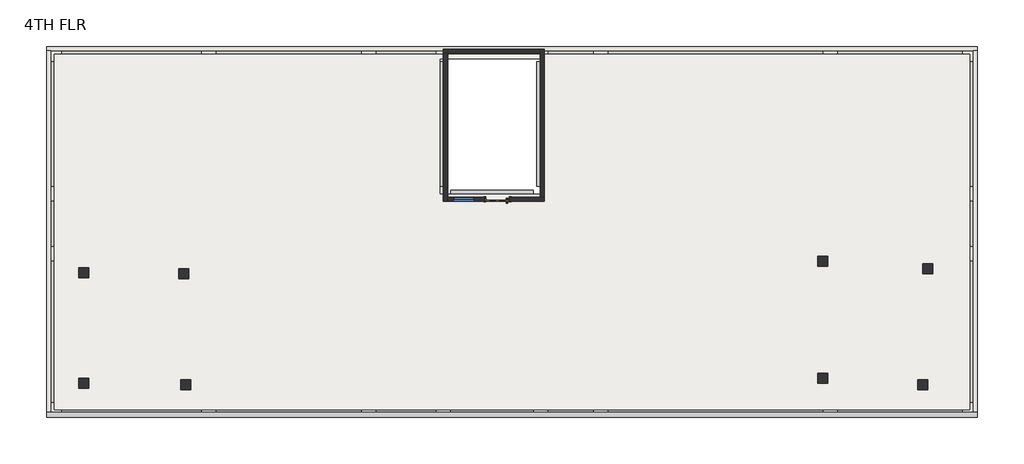
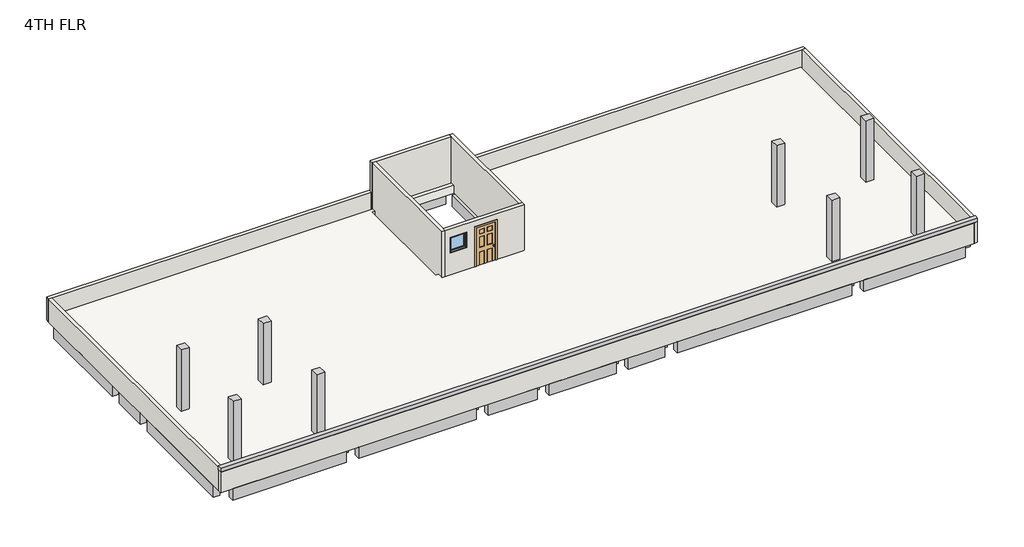
# One storey: 52 beams, 8 columns, 8 walls, 1 door, 1 proxy, 1 roof, 1 window.
"""IFC4 building model written with IfcOpenShell, lengths in millimetres."""

from ifc_helpers import new_model, si_unit, frame, origin, place, context, project, spatial, polyline, outline, extrude, faceted_brep, transform, mapped, element, save
from components import rectangular_column_1_x_1_column_3bfae6ee, door_56a52d02, window_d757e824

model = new_model("IFC4")

# Units and contexts
model_context = context("Model", 3, world=origin())
ifc_project = project(units=[si_unit("LENGTHUNIT", "METRE", prefix="MILLI")], contexts=[model_context])

# Site, building, storey
site = spatial("IfcSite", under=ifc_project)
building = spatial("IfcBuilding", under=site)
storey = spatial("IfcBuildingStorey", under=building, Name="4TH FLR", Elevation=12496.8)

# Beams
placement = place(None, origin())
element("IfcBeam", 1, ObjectType="Concrete-Rectangular Beam : 9\" X 18\" BEAM", at=placement, inside=storey, context=model_context, shape_type="SweptSolid", body=[
    extrude(outline(polyline([(-10649.5456086, -10887.8679047), (-10649.5456086, -11116.4679047), (-14916.7456086, -11116.4679047), (-14916.7456086, -10887.8679047), (-10649.5456086, -10887.8679047)])), frame((0.0, 0.0, 12039.6), z_axis=(0.0, 0.0, 1.0), x_axis=(1.0, 0.0, 0.0)), (0.0, 0.0, 1.0), 457.2),
])
element("IfcBeam", 2, ObjectType="Concrete-Rectangular Beam : 9\" X 18\" BEAM", at=placement, inside=storey, context=model_context, shape_type="SweptSolid", body=[
    extrude(outline(polyline([(-5772.7456086, -10887.8679047), (-5772.7456086, -11116.4679047), (-10192.3456086, -11116.4679047), (-10192.3456086, -10887.8679047), (-5772.7456086, -10887.8679047)])), frame((0.0, 0.0, 12039.6), z_axis=(0.0, 0.0, 1.0), x_axis=(1.0, 0.0, 0.0)), (0.0, 0.0, 1.0), 457.2),
])
element("IfcBeam", 3, ObjectType="Concrete-Rectangular Beam : 9\" X 18\" BEAM", at=placement, inside=storey, context=model_context, shape_type="SweptSolid", body=[
    extrude(outline(polyline([(-3486.7456086, -10887.8679047), (-3486.7456086, -11116.4679047), (-5315.5456086, -11116.4679047), (-5315.5456086, -10887.8679047), (-3486.7456086, -10887.8679047)])), frame((0.0, 0.0, 12039.6), z_axis=(0.0, 0.0, 1.0), x_axis=(1.0, 0.0, 0.0)), (0.0, 0.0, 1.0), 457.2),
])
element("IfcBeam", 4, ObjectType="Concrete-Rectangular Beam : 9\" X 18\" BEAM", at=placement, inside=storey, context=model_context, shape_type="SweptSolid", body=[
    extrude(outline(polyline([(-518.4083398, -10887.8679047), (-518.4083398, -11116.4679047), (-3029.5456086, -11116.4679047), (-3029.5456086, -10887.8679047), (-518.4083398, -10887.8679047)])), frame((0.0, 0.0, 12039.6), z_axis=(0.0, 0.0, 1.0), x_axis=(1.0, 0.0, 0.0)), (0.0, 0.0, 1.0), 457.2),
])
element("IfcBeam", 5, ObjectType="Concrete-Rectangular Beam : 9\" X 18\" BEAM", at=placement, inside=storey, context=model_context, shape_type="SweptSolid", body=[
    extrude(outline(polyline([(1310.3916602, -10887.8679047), (1310.3916602, -11116.4679047), (-61.2083398, -11116.4679047), (-61.2083398, -10887.8679047), (1310.3916602, -10887.8679047)])), frame((0.0, 0.0, 12039.6), z_axis=(0.0, 0.0, 1.0), x_axis=(1.0, 0.0, 0.0)), (0.0, 0.0, 1.0), 457.2),
])
element("IfcBeam", 6, ObjectType="Concrete-Rectangular Beam : 9\" X 18\" BEAM", at=placement, inside=storey, context=model_context, shape_type="SweptSolid", body=[
    extrude(outline(polyline([(1424.6916602, -6358.3794704), (1653.2916602, -6358.3794704), (1653.2916602, -10659.2679047), (1424.6916602, -10659.2679047), (1424.6916602, -6358.3794704)])), frame((0.0, 0.0, 12039.6), z_axis=(0.0, 0.0, 1.0), x_axis=(1.0, 0.0, 0.0)), (0.0, 0.0, 1.0), 457.2),
])
element("IfcBeam", 7, ObjectType="Concrete-Rectangular Beam : 9\" X 18\" BEAM", at=placement, inside=storey, context=model_context, shape_type="SweptSolid", body=[
    extrude(outline(polyline([(1424.6916602, -4529.5794704), (1653.2916602, -4529.5794704), (1653.2916602, -5901.1794704), (1424.6916602, -5901.1794704), (1424.6916602, -4529.5794704)])), frame((0.0, 0.0, 12039.6), z_axis=(0.0, 0.0, 1.0), x_axis=(1.0, 0.0, 0.0)), (0.0, 0.0, 1.0), 457.2),
])
element("IfcBeam", 8, ObjectType="Concrete-Rectangular Beam : 9\" X 18\" BEAM", at=placement, inside=storey, context=model_context, shape_type="SweptSolid", body=[
    extrude(outline(polyline([(8317.2128058, -10887.8679047), (8317.2128058, -11116.4679047), (1767.5916602, -11116.4679047), (1767.5916602, -10887.8679047), (8317.2128058, -10887.8679047)])), frame((0.0, 0.0, 12039.6), z_axis=(0.0, 0.0, 1.0), x_axis=(1.0, 0.0, 0.0)), (0.0, 0.0, 1.0), 457.2),
])
element("IfcBeam", 9, ObjectType="Concrete-Rectangular Beam : 9\" X 18\" BEAM", at=placement, inside=storey, context=model_context, shape_type="SweptSolid", body=[
    extrude(outline(polyline([(12584.4128058, -10887.8679047), (12584.4128058, -11116.4679047), (8774.4128058, -11116.4679047), (8774.4128058, -10887.8679047), (12584.4128058, -10887.8679047)])), frame((0.0, 0.0, 12039.6), z_axis=(0.0, 0.0, 1.0), x_axis=(1.0, 0.0, 0.0)), (0.0, 0.0, 1.0), 457.2),
])
element("IfcBeam", 10, ObjectType="Concrete-Rectangular Beam : 9\" X 18\" BEAM", at=placement, inside=storey, context=model_context, shape_type="SweptSolid", body=[
    extrude(outline(polyline([(12813.0128058, -6358.3794704), (13041.6128058, -6358.3794704), (13041.6128058, -10659.2679047), (12813.0128058, -10659.2679047), (12813.0128058, -6358.3794704)])), frame((0.0, 0.0, 12039.6), z_axis=(0.0, 0.0, 1.0), x_axis=(1.0, 0.0, 0.0)), (0.0, 0.0, 1.0), 457.2),
])
element("IfcBeam", 11, ObjectType="Concrete-Rectangular Beam : 9\" X 18\" BEAM", at=placement, inside=storey, context=model_context, shape_type="SweptSolid", body=[
    extrude(outline(polyline([(12813.0128058, -4529.5794704), (13041.6128058, -4529.5794704), (13041.6128058, -5901.1794704), (12813.0128058, -5901.1794704), (12813.0128058, -4529.5794704)])), frame((0.0, 0.0, 12039.6), z_axis=(0.0, 0.0, 1.0), x_axis=(1.0, 0.0, 0.0)), (0.0, 0.0, 1.0), 457.2),
])
element("IfcBeam", 12, ObjectType="Concrete-Rectangular Beam : 9\" X 18\" BEAM", at=placement, inside=storey, context=model_context, shape_type="SweptSolid", body=[
    extrude(outline(polyline([(12813.0128058, -262.3794704), (13041.6128058, -262.3794704), (13041.6128058, -4072.3794704), (12813.0128058, -4072.3794704), (12813.0128058, -262.3794704)])), frame((0.0, 0.0, 12039.6), z_axis=(0.0, 0.0, 1.0), x_axis=(1.0, 0.0, 0.0)), (0.0, 0.0, 1.0), 457.2),
])
element("IfcBeam", 13, ObjectType="Concrete-Rectangular Beam : 9\" X 18\" BEAM", at=placement, inside=storey, context=model_context, shape_type="SweptSolid", body=[
    extrude(outline(polyline([(8774.4128058, -33.7794704), (8774.4128058, 194.8205296), (12584.4128058, 194.8205296), (12584.4128058, -33.7794704), (8774.4128058, -33.7794704)])), frame((0.0, 0.0, 12039.6), z_axis=(0.0, 0.0, 1.0), x_axis=(1.0, 0.0, 0.0)), (0.0, 0.0, 1.0), 457.2),
])
element("IfcBeam", 14, ObjectType="Concrete-Rectangular Beam : 9\" X 18\" BEAM", at=placement, inside=storey, context=model_context, shape_type="SweptSolid", body=[
    extrude(outline(polyline([(1767.5916602, -33.7794704), (1767.5916602, 194.8205296), (8317.2128058, 194.8205296), (8317.2128058, -33.7794704), (1767.5916602, -33.7794704)])), frame((0.0, 0.0, 12039.6), z_axis=(0.0, 0.0, 1.0), x_axis=(1.0, 0.0, 0.0)), (0.0, 0.0, 1.0), 457.2),
])
element("IfcBeam", 15, ObjectType="Concrete-Rectangular Beam : 9\" X 18\" BEAM", at=placement, inside=storey, context=model_context, shape_type="SweptSolid", body=[
    extrude(outline(polyline([(-61.2083398, -33.7794704), (-61.2083398, 194.8205296), (1310.3916602, 194.8205296), (1310.3916602, -33.7794704), (-61.2083398, -33.7794704)])), frame((0.0, 0.0, 12039.6), z_axis=(0.0, 0.0, 1.0), x_axis=(1.0, 0.0, 0.0)), (0.0, 0.0, 1.0), 457.2),
])
element("IfcBeam", 16, ObjectType="Concrete-Rectangular Beam : 9\" X 18\" BEAM", at=placement, inside=storey, context=model_context, shape_type="SweptSolid", body=[
    extrude(outline(polyline([(-3029.5456086, -33.7794704), (-3029.5456086, 194.8205296), (-518.4083398, 194.8205296), (-518.4083398, -33.7794704), (-3029.5456086, -33.7794704)])), frame((0.0, 0.0, 12039.6), z_axis=(0.0, 0.0, 1.0), x_axis=(1.0, 0.0, 0.0)), (0.0, 0.0, 1.0), 457.2),
])
element("IfcBeam", 17, ObjectType="Concrete-Rectangular Beam : 9\" X 18\" BEAM", at=placement, inside=storey, context=model_context, shape_type="SweptSolid", body=[
    extrude(outline(polyline([(-5315.5456086, -33.7794704), (-5315.5456086, 194.8205296), (-3486.7456086, 194.8205296), (-3486.7456086, -33.7794704), (-5315.5456086, -33.7794704)])), frame((0.0, 0.0, 12039.6), z_axis=(0.0, 0.0, 1.0), x_axis=(1.0, 0.0, 0.0)), (0.0, 0.0, 1.0), 457.2),
])
element("IfcBeam", 18, ObjectType="Concrete-Rectangular Beam : 9\" X 18\" BEAM", at=placement, inside=storey, context=model_context, shape_type="SweptSolid", body=[
    extrude(outline(polyline([(-10192.3456086, -33.7794704), (-10192.3456086, 194.8205296), (-5772.7456086, 194.8205296), (-5772.7456086, -33.7794704), (-10192.3456086, -33.7794704)])), frame((0.0, 0.0, 12039.6), z_axis=(0.0, 0.0, 1.0), x_axis=(1.0, 0.0, 0.0)), (0.0, 0.0, 1.0), 457.2),
])
element("IfcBeam", 19, ObjectType="Concrete-Rectangular Beam : 9\" X 18\" BEAM", at=placement, inside=storey, context=model_context, shape_type="SweptSolid", body=[
    extrude(outline(polyline([(-14916.7456086, -33.7794704), (-14916.7456086, 194.8205296), (-10649.5456086, 194.8205296), (-10649.5456086, -33.7794704), (-14916.7456086, -33.7794704)])), frame((0.0, 0.0, 12039.6), z_axis=(0.0, 0.0, 1.0), x_axis=(1.0, 0.0, 0.0)), (0.0, 0.0, 1.0), 457.2),
])
element("IfcBeam", 20, ObjectType="Concrete-Rectangular Beam : 9\" X 18\" BEAM", at=placement, inside=storey, context=model_context, shape_type="SweptSolid", body=[
    extrude(outline(polyline([(-15145.3456086, -4072.3794704), (-15373.9456086, -4072.3794704), (-15373.9456086, -262.3794704), (-15145.3456086, -262.3794704), (-15145.3456086, -4072.3794704)])), frame((0.0, 0.0, 12039.6), z_axis=(0.0, 0.0, 1.0), x_axis=(1.0, 0.0, 0.0)), (0.0, 0.0, 1.0), 457.2),
])
element("IfcBeam", 21, ObjectType="Concrete-Rectangular Beam : 9\" X 18\" BEAM", at=placement, inside=storey, context=model_context, shape_type="SweptSolid", body=[
    extrude(outline(polyline([(-15145.3456086, -5901.1794704), (-15373.9456086, -5901.1794704), (-15373.9456086, -4529.5794704), (-15145.3456086, -4529.5794704), (-15145.3456086, -5901.1794704)])), frame((0.0, 0.0, 12039.6), z_axis=(0.0, 0.0, 1.0), x_axis=(1.0, 0.0, 0.0)), (0.0, 0.0, 1.0), 457.2),
])
element("IfcBeam", 22, ObjectType="Concrete-Rectangular Beam : 9\" X 18\" BEAM", at=placement, inside=storey, context=model_context, shape_type="SweptSolid", body=[
    extrude(outline(polyline([(-15145.3456086, -10659.2679047), (-15373.9456086, -10659.2679047), (-15373.9456086, -6358.3794704), (-15145.3456086, -6358.3794704), (-15145.3456086, -10659.2679047)])), frame((0.0, 0.0, 12039.6), z_axis=(0.0, 0.0, 1.0), x_axis=(1.0, 0.0, 0.0)), (0.0, 0.0, 1.0), 457.2),
])
element("IfcBeam", 23, ObjectType="Concrete-Rectangular Beam : 9\" X 18\" BEAM", at=placement, inside=storey, context=model_context, shape_type="SweptSolid", body=[
    extrude(outline(polyline([(-10649.5456086, -4186.6794704), (-10649.5456086, -4415.2794704), (-14916.7456086, -4415.2794704), (-14916.7456086, -4186.6794704), (-10649.5456086, -4186.6794704)])), frame((0.0, 0.0, 12039.6), z_axis=(0.0, 0.0, 1.0), x_axis=(1.0, 0.0, 0.0)), (0.0, 0.0, 1.0), 457.2),
])
element("IfcBeam", 24, ObjectType="Concrete-Rectangular Beam : 9\" X 18\" BEAM", at=placement, inside=storey, context=model_context, shape_type="SweptSolid", body=[
    extrude(outline(polyline([(-5772.7456086, -4186.6794704), (-5772.7456086, -4415.2794704), (-10192.3456086, -4415.2794704), (-10192.3456086, -4186.6794704), (-5772.7456086, -4186.6794704)])), frame((0.0, 0.0, 12039.6), z_axis=(0.0, 0.0, 1.0), x_axis=(1.0, 0.0, 0.0)), (0.0, 0.0, 1.0), 457.2),
])
element("IfcBeam", 25, ObjectType="Concrete-Rectangular Beam : 9\" X 18\" BEAM", at=placement, inside=storey, context=model_context, shape_type="SweptSolid", body=[
    extrude(outline(polyline([(-3486.7456086, -4186.6794704), (-3486.7456086, -4415.2794704), (-5315.5456086, -4415.2794704), (-5315.5456086, -4186.6794704), (-3486.7456086, -4186.6794704)])), frame((0.0, 0.0, 12039.6), z_axis=(0.0, 0.0, 1.0), x_axis=(1.0, 0.0, 0.0)), (0.0, 0.0, 1.0), 457.2),
])
element("IfcBeam", 26, ObjectType="Concrete-Rectangular Beam : 9\" X 18\" BEAM", at=placement, inside=storey, context=model_context, shape_type="SweptSolid", body=[
    extrude(outline(polyline([(-518.4083398, -4186.6794704), (-518.4083398, -4415.2794704), (-3029.5456086, -4415.2794704), (-3029.5456086, -4186.6794704), (-518.4083398, -4186.6794704)])), frame((0.0, 0.0, 12039.6), z_axis=(0.0, 0.0, 1.0), x_axis=(1.0, 0.0, 0.0)), (0.0, 0.0, 1.0), 457.2),
])
element("IfcBeam", 27, ObjectType="Concrete-Rectangular Beam : 9\" X 18\" BEAM", at=placement, inside=storey, context=model_context, shape_type="SweptSolid", body=[
    extrude(outline(polyline([(1310.3916602, -4186.6794704), (1310.3916602, -4415.2794704), (-61.2083398, -4415.2794704), (-61.2083398, -4186.6794704), (1310.3916602, -4186.6794704)])), frame((0.0, 0.0, 12039.6), z_axis=(0.0, 0.0, 1.0), x_axis=(1.0, 0.0, 0.0)), (0.0, 0.0, 1.0), 457.2),
])
element("IfcBeam", 28, ObjectType="Concrete-Rectangular Beam : 9\" X 18\" BEAM", at=placement, inside=storey, context=model_context, shape_type="SweptSolid", body=[
    extrude(outline(polyline([(1424.6916602, -262.3794704), (1653.2916602, -262.3794704), (1653.2916602, -4072.3794704), (1424.6916602, -4072.3794704), (1424.6916602, -262.3794704)])), frame((0.0, 0.0, 12039.6), z_axis=(0.0, 0.0, 1.0), x_axis=(1.0, 0.0, 0.0)), (0.0, 0.0, 1.0), 457.2),
])
element("IfcBeam", 29, ObjectType="Concrete-Rectangular Beam : 9\" X 18\" BEAM", at=placement, inside=storey, context=model_context, shape_type="SweptSolid", body=[
    extrude(outline(polyline([(-175.5083398, -4072.3794704), (-404.1083398, -4072.3794704), (-404.1083398, -262.3794704), (-175.5083398, -262.3794704), (-175.5083398, -4072.3794704)])), frame((0.0, 0.0, 12039.6), z_axis=(0.0, 0.0, 1.0), x_axis=(1.0, 0.0, 0.0)), (0.0, 0.0, 1.0), 457.2),
])
element("IfcBeam", 30, ObjectType="Concrete-Rectangular Beam : 9\" X 18\" BEAM", at=placement, inside=storey, context=model_context, shape_type="SweptSolid", body=[
    extrude(outline(polyline([(-3143.8456086, -4072.3794704), (-3372.4456086, -4072.3794704), (-3372.4456086, -262.3794704), (-3143.8456086, -262.3794704), (-3143.8456086, -4072.3794704)])), frame((0.0, 0.0, 12039.6), z_axis=(0.0, 0.0, 1.0), x_axis=(1.0, 0.0, 0.0)), (0.0, 0.0, 1.0), 457.2),
])
element("IfcBeam", 31, ObjectType="Concrete-Rectangular Beam : 9\" X 18\" BEAM", at=placement, inside=storey, context=model_context, shape_type="SweptSolid", body=[
    extrude(outline(polyline([(-5429.8456086, -4072.3794704), (-5658.4456086, -4072.3794704), (-5658.4456086, -262.3794704), (-5429.8456086, -262.3794704), (-5429.8456086, -4072.3794704)])), frame((0.0, 0.0, 12039.6), z_axis=(0.0, 0.0, 1.0), x_axis=(1.0, 0.0, 0.0)), (0.0, 0.0, 1.0), 457.2),
])
element("IfcBeam", 32, ObjectType="Concrete-Rectangular Beam : 9\" X 18\" BEAM", at=placement, inside=storey, context=model_context, shape_type="SweptSolid", body=[
    extrude(outline(polyline([(-10306.6456086, -4072.3794704), (-10535.2456086, -4072.3794704), (-10535.2456086, -262.3794704), (-10306.6456086, -262.3794704), (-10306.6456086, -4072.3794704)])), frame((0.0, 0.0, 12039.6), z_axis=(0.0, 0.0, 1.0), x_axis=(1.0, 0.0, 0.0)), (0.0, 0.0, 1.0), 457.2),
])
element("IfcBeam", 33, ObjectType="Concrete-Rectangular Beam : 9\" X 18\" BEAM", at=placement, inside=storey, context=model_context, shape_type="SweptSolid", body=[
    extrude(outline(polyline([(-10649.5456086, -6015.4794704), (-10649.5456086, -6244.0794704), (-14916.7456086, -6244.0794704), (-14916.7456086, -6015.4794704), (-10649.5456086, -6015.4794704)])), frame((0.0, 0.0, 12039.6), z_axis=(0.0, 0.0, 1.0), x_axis=(1.0, 0.0, 0.0)), (0.0, 0.0, 1.0), 457.2),
])
element("IfcBeam", 34, ObjectType="Concrete-Rectangular Beam : 9\" X 18\" BEAM", at=placement, inside=storey, context=model_context, shape_type="SweptSolid", body=[
    extrude(outline(polyline([(-5772.7456086, -6015.4794704), (-5772.7456086, -6244.0794704), (-10192.3456086, -6244.0794704), (-10192.3456086, -6015.4794704), (-5772.7456086, -6015.4794704)])), frame((0.0, 0.0, 12039.6), z_axis=(0.0, 0.0, 1.0), x_axis=(1.0, 0.0, 0.0)), (0.0, 0.0, 1.0), 457.2),
])
element("IfcBeam", 35, ObjectType="Concrete-Rectangular Beam : 9\" X 18\" BEAM", at=placement, inside=storey, context=model_context, shape_type="SweptSolid", body=[
    extrude(outline(polyline([(-3486.7456086, -6015.4794704), (-3486.7456086, -6244.0794704), (-5315.5456086, -6244.0794704), (-5315.5456086, -6015.4794704), (-3486.7456086, -6015.4794704)])), frame((0.0, 0.0, 12039.6), z_axis=(0.0, 0.0, 1.0), x_axis=(1.0, 0.0, 0.0)), (0.0, 0.0, 1.0), 457.2),
])
element("IfcBeam", 36, ObjectType="Concrete-Rectangular Beam : 9\" X 18\" BEAM", at=placement, inside=storey, context=model_context, shape_type="SweptSolid", body=[
    extrude(outline(polyline([(-3029.5456086, -6244.0794704), (-3029.5456086, -6015.4794704), (-518.4083398, -6015.4794704), (-518.4083398, -6244.0794704), (-3029.5456086, -6244.0794704)])), frame((0.0, 0.0, 12039.6), z_axis=(0.0, 0.0, 1.0), x_axis=(1.0, 0.0, 0.0)), (0.0, 0.0, 1.0), 457.2),
])
element("IfcBeam", 37, ObjectType="Concrete-Rectangular Beam : 9\" X 18\" BEAM", at=placement, inside=storey, context=model_context, shape_type="SweptSolid", body=[
    extrude(outline(polyline([(1310.3916602, -6015.4794704), (1310.3916602, -6244.0794704), (-61.2083398, -6244.0794704), (-61.2083398, -6015.4794704), (1310.3916602, -6015.4794704)])), frame((0.0, 0.0, 12039.6), z_axis=(0.0, 0.0, 1.0), x_axis=(1.0, 0.0, 0.0)), (0.0, 0.0, 1.0), 457.2),
])
element("IfcBeam", 38, ObjectType="Concrete-Rectangular Beam : 9\" X 18\" BEAM", at=placement, inside=storey, context=model_context, shape_type="SweptSolid", body=[
    extrude(outline(polyline([(-10535.2456086, -6358.3794704), (-10306.6456086, -6358.3794704), (-10306.6456086, -10659.2679047), (-10535.2456086, -10659.2679047), (-10535.2456086, -6358.3794704)])), frame((0.0, 0.0, 12039.6), z_axis=(0.0, 0.0, 1.0), x_axis=(1.0, 0.0, 0.0)), (0.0, 0.0, 1.0), 457.2),
])
element("IfcBeam", 39, ObjectType="Concrete-Rectangular Beam : 9\" X 18\" BEAM", at=placement, inside=storey, context=model_context, shape_type="SweptSolid", body=[
    extrude(outline(polyline([(-5658.4456086, -6358.3794704), (-5429.8456086, -6358.3794704), (-5429.8456086, -10659.2679047), (-5658.4456086, -10659.2679047), (-5658.4456086, -6358.3794704)])), frame((0.0, 0.0, 12039.6), z_axis=(0.0, 0.0, 1.0), x_axis=(1.0, 0.0, 0.0)), (0.0, 0.0, 1.0), 457.2),
])
element("IfcBeam", 40, ObjectType="Concrete-Rectangular Beam : 9\" X 18\" BEAM", at=placement, inside=storey, context=model_context, shape_type="SweptSolid", body=[
    extrude(outline(polyline([(-3372.4456086, -6358.3794704), (-3143.8456086, -6358.3794704), (-3143.8456086, -10659.2679047), (-3372.4456086, -10659.2679047), (-3372.4456086, -6358.3794704)])), frame((0.0, 0.0, 12039.6), z_axis=(0.0, 0.0, 1.0), x_axis=(1.0, 0.0, 0.0)), (0.0, 0.0, 1.0), 457.2),
])
element("IfcBeam", 41, ObjectType="Concrete-Rectangular Beam : 9\" X 18\" BEAM", at=placement, inside=storey, context=model_context, shape_type="SweptSolid", body=[
    extrude(outline(polyline([(-404.1083398, -6358.3794704), (-175.5083398, -6358.3794704), (-175.5083398, -10659.2679047), (-404.1083398, -10659.2679047), (-404.1083398, -6358.3794704)])), frame((0.0, 0.0, 12039.6), z_axis=(0.0, 0.0, 1.0), x_axis=(1.0, 0.0, 0.0)), (0.0, 0.0, 1.0), 457.2),
])
element("IfcBeam", 42, ObjectType="Concrete-Rectangular Beam : 9\" X 18\" BEAM", at=placement, inside=storey, context=model_context, shape_type="SweptSolid", body=[
    extrude(outline(polyline([(-404.1083398, -4529.5794704), (-175.5083398, -4529.5794704), (-175.5083398, -5901.1794704), (-404.1083398, -5901.1794704), (-404.1083398, -4529.5794704)])), frame((0.0, 0.0, 12039.6), z_axis=(0.0, 0.0, 1.0), x_axis=(1.0, 0.0, 0.0)), (0.0, 0.0, 1.0), 457.2),
])
element("IfcBeam", 43, ObjectType="Concrete-Rectangular Beam : 9\" X 18\" BEAM", at=placement, inside=storey, context=model_context, shape_type="SweptSolid", body=[
    extrude(outline(polyline([(-3143.8456086, -5901.1794704), (-3372.4456086, -5901.1794704), (-3372.4456086, -4529.5794704), (-3143.8456086, -4529.5794704), (-3143.8456086, -5901.1794704)])), frame((0.0, 0.0, 12039.6), z_axis=(0.0, 0.0, 1.0), x_axis=(1.0, 0.0, 0.0)), (0.0, 0.0, 1.0), 457.2),
])
element("IfcBeam", 44, ObjectType="Concrete-Rectangular Beam : 9\" X 18\" BEAM", at=placement, inside=storey, context=model_context, shape_type="SweptSolid", body=[
    extrude(outline(polyline([(-5429.8456086, -5901.1794704), (-5658.4456086, -5901.1794704), (-5658.4456086, -4529.5794704), (-5429.8456086, -4529.5794704), (-5429.8456086, -5901.1794704)])), frame((0.0, 0.0, 12039.6), z_axis=(0.0, 0.0, 1.0), x_axis=(1.0, 0.0, 0.0)), (0.0, 0.0, 1.0), 457.2),
])
element("IfcBeam", 45, ObjectType="Concrete-Rectangular Beam : 9\" X 18\" BEAM", at=placement, inside=storey, context=model_context, shape_type="SweptSolid", body=[
    extrude(outline(polyline([(-10306.6456086, -5901.1794704), (-10535.2456086, -5901.1794704), (-10535.2456086, -4529.5794704), (-10306.6456086, -4529.5794704), (-10306.6456086, -5901.1794704)])), frame((0.0, 0.0, 12039.6), z_axis=(0.0, 0.0, 1.0), x_axis=(1.0, 0.0, 0.0)), (0.0, 0.0, 1.0), 457.2),
])
element("IfcBeam", 46, ObjectType="Concrete-Rectangular Beam : 9\" X 18\" BEAM", at=placement, inside=storey, context=model_context, shape_type="SweptSolid", body=[
    extrude(outline(polyline([(8317.2128058, -4186.6794704), (8317.2128058, -4415.2794704), (1767.5916602, -4415.2794704), (1767.5916602, -4186.6794704), (8317.2128058, -4186.6794704)])), frame((0.0, 0.0, 12039.6), z_axis=(0.0, 0.0, 1.0), x_axis=(1.0, 0.0, 0.0)), (0.0, 0.0, 1.0), 457.2),
])
element("IfcBeam", 47, ObjectType="Concrete-Rectangular Beam : 9\" X 18\" BEAM", at=placement, inside=storey, context=model_context, shape_type="SweptSolid", body=[
    extrude(outline(polyline([(12584.4128058, -4186.6794704), (12584.4128058, -4415.2794704), (8774.4128058, -4415.2794704), (8774.4128058, -4186.6794704), (12584.4128058, -4186.6794704)])), frame((0.0, 0.0, 12039.6), z_axis=(0.0, 0.0, 1.0), x_axis=(1.0, 0.0, 0.0)), (0.0, 0.0, 1.0), 457.2),
])
element("IfcBeam", 48, ObjectType="Concrete-Rectangular Beam : 9\" X 18\" BEAM", at=placement, inside=storey, context=model_context, shape_type="SweptSolid", body=[
    extrude(outline(polyline([(8774.4128058, -6244.0794704), (8774.4128058, -6015.4794704), (12584.4128058, -6015.4794704), (12584.4128058, -6244.0794704), (8774.4128058, -6244.0794704)])), frame((0.0, 0.0, 12039.6), z_axis=(0.0, 0.0, 1.0), x_axis=(1.0, 0.0, 0.0)), (0.0, 0.0, 1.0), 457.2),
])
element("IfcBeam", 49, ObjectType="Concrete-Rectangular Beam : 9\" X 18\" BEAM", at=placement, inside=storey, context=model_context, shape_type="SweptSolid", body=[
    extrude(outline(polyline([(1767.5916602, -6244.0794704), (1767.5916602, -6015.4794704), (8317.2128058, -6015.4794704), (8317.2128058, -6244.0794704), (1767.5916602, -6244.0794704)])), frame((0.0, 0.0, 12039.6), z_axis=(0.0, 0.0, 1.0), x_axis=(1.0, 0.0, 0.0)), (0.0, 0.0, 1.0), 457.2),
])
element("IfcBeam", 50, ObjectType="Concrete-Rectangular Beam : 9\" X 18\" BEAM", at=placement, inside=storey, context=model_context, shape_type="SweptSolid", body=[
    extrude(outline(polyline([(8431.5128058, -6358.3794704), (8660.1128058, -6358.3794704), (8660.1128058, -10659.2679047), (8431.5128058, -10659.2679047), (8431.5128058, -6358.3794704)])), frame((0.0, 0.0, 12039.6), z_axis=(0.0, 0.0, 1.0), x_axis=(1.0, 0.0, 0.0)), (0.0, 0.0, 1.0), 457.2),
])
element("IfcBeam", 51, ObjectType="Concrete-Rectangular Beam : 9\" X 18\" BEAM", at=placement, inside=storey, context=model_context, shape_type="SweptSolid", body=[
    extrude(outline(polyline([(8431.5128058, -4529.5794704), (8660.1128058, -4529.5794704), (8660.1128058, -5901.1794704), (8431.5128058, -5901.1794704), (8431.5128058, -4529.5794704)])), frame((0.0, 0.0, 12039.6), z_axis=(0.0, 0.0, 1.0), x_axis=(1.0, 0.0, 0.0)), (0.0, 0.0, 1.0), 457.2),
])
element("IfcBeam", 52, ObjectType="Concrete-Rectangular Beam : 9\" X 18\" BEAM", at=placement, inside=storey, context=model_context, shape_type="SweptSolid", body=[
    extrude(outline(polyline([(8431.5128058, -262.3794704), (8660.1128058, -262.3794704), (8660.1128058, -4072.3794704), (8431.5128058, -4072.3794704), (8431.5128058, -262.3794704)])), frame((0.0, 0.0, 12039.6), z_axis=(0.0, 0.0, 1.0), x_axis=(1.0, 0.0, 0.0)), (0.0, 0.0, 1.0), 457.2),
])

# Proxy
element("IfcBuildingElementProxy", 53, Name="Reveal", ObjectType="Reveal", at=placement, inside=storey, context=model_context, shape_type="SweptSolid", body=[
    extrude(outline(polyline([(13041.6128058, -10964.0679047), (13041.6128058, -11116.4679047), (-15373.9456086, -11116.4679047), (-15373.9456086, -10964.0679047), (13041.6128058, -10964.0679047)])), frame((0.0, 0.0, 13309.6), z_axis=(0.0, 0.0, 1.0), x_axis=(1.0, 0.0, 0.0)), (0.0, 0.0, 1.0), 152.4),
])

# Columns
rectangular_column_1_x_1_column_shape = rectangular_column_1_x_1_column_3bfae6ee(model_context)
element("IfcColumn", 54, ObjectType="Rectangular Column : 1' X 1' COLUMN", at=placement, inside=storey, context=model_context, shape_type="MappedRepresentation", body=[
    mapped(rectangular_column_1_x_1_column_shape, transform((-14242.4401855, -10087.7679047, 0.0), x_axis=(1.0, 0.0, 0.0), y_axis=(0.0, 1.0, 0.0), z_axis=(0.0, 0.0, 1.0))),
])
element("IfcColumn", 55, ObjectType="Rectangular Column : 1' X 1' COLUMN", at=placement, inside=storey, context=model_context, shape_type="MappedRepresentation", body=[
    mapped(rectangular_column_1_x_1_column_shape, transform((-14242.4401855, -6713.9794704, 0.0), x_axis=(1.0, 0.0, 0.0), y_axis=(0.0, 1.0, 0.0), z_axis=(0.0, 0.0, 1.0))),
])
element("IfcColumn", 56, ObjectType="Rectangular Column : 1' X 1' COLUMN", at=placement, inside=storey, context=model_context, shape_type="MappedRepresentation", body=[
    mapped(rectangular_column_1_x_1_column_shape, transform((-11182.9456086, -6739.3794704, 0.0), x_axis=(1.0, 0.0, 0.0), y_axis=(0.0, 1.0, 0.0), z_axis=(0.0, 0.0, 1.0))),
])
element("IfcColumn", 57, ObjectType="Rectangular Column : 1' X 1' COLUMN", at=placement, inside=storey, context=model_context, shape_type="MappedRepresentation", body=[
    mapped(rectangular_column_1_x_1_column_shape, transform((-11132.1456086, -10125.8679047, 0.0), x_axis=(1.0, 0.0, 0.0), y_axis=(0.0, 1.0, 0.0), z_axis=(0.0, 0.0, 1.0))),
])
element("IfcColumn", 58, ObjectType="Rectangular Column : 1' X 1' COLUMN", at=placement, inside=storey, context=model_context, shape_type="MappedRepresentation", body=[
    mapped(rectangular_column_1_x_1_column_shape, transform((8312.7598145, -9935.3679047, 0.0), x_axis=(1.0, 0.0, 0.0), y_axis=(0.0, 1.0, 0.0), z_axis=(0.0, 0.0, 1.0))),
])
element("IfcColumn", 59, ObjectType="Rectangular Column : 1' X 1' COLUMN", at=placement, inside=storey, context=model_context, shape_type="MappedRepresentation", body=[
    mapped(rectangular_column_1_x_1_column_shape, transform((8312.7598145, -6358.3794704, 0.0), x_axis=(1.0, 0.0, 0.0), y_axis=(0.0, 1.0, 0.0), z_axis=(0.0, 0.0, 1.0))),
])
element("IfcColumn", 60, ObjectType="Rectangular Column : 1' X 1' COLUMN", at=placement, inside=storey, context=model_context, shape_type="MappedRepresentation", body=[
    mapped(rectangular_column_1_x_1_column_shape, transform((11524.6543914, -6586.9794704, 0.0), x_axis=(1.0, 0.0, 0.0), y_axis=(0.0, 1.0, 0.0), z_axis=(0.0, 0.0, 1.0))),
])
element("IfcColumn", 61, ObjectType="Rectangular Column : 1' X 1' COLUMN", at=placement, inside=storey, context=model_context, shape_type="MappedRepresentation", body=[
    mapped(rectangular_column_1_x_1_column_shape, transform((11372.2543914, -10125.8679047, 0.0), x_axis=(1.0, 0.0, 0.0), y_axis=(0.0, 1.0, 0.0), z_axis=(0.0, 0.0, 1.0))),
])

# Door
door_shape = door_56a52d02(model_context)
element("IfcDoor", 62, ObjectType="Door-Interior-Single-6_Panel-Wood : 2'4\" X 6'", at=placement, inside=storey, context=model_context, shape_type="MappedRepresentation", body=[
    mapped(door_shape, transform((-1610.6083398, -4469.2544704, 12496.8), x_axis=(-1.0, 0.0, 0.0), y_axis=(0.0, -1.0, 0.0), z_axis=(0.0, 0.0, 1.0))),
])

# Roof
element("IfcRoof", 63, ObjectType="Generic - 12\"", at=placement, inside=storey, context=model_context, shape_type="SweptSolid", body=[
    extrude(outline(polyline([(12813.0128058, -10887.8679047), (-15145.3456086, -10887.8679047), (-15145.3456086, -33.7794704), (12813.0128058, -33.7794704), (12813.0128058, -10887.8679047)]), holes=[polyline([(-289.8083398, -186.1794704), (-3359.7456086, -186.1794704), (-3359.7456086, -4300.9794704), (-289.8083398, -4300.9794704), (-289.8083398, -186.1794704)])]), frame((0.0, 0.0, 12496.8), z_axis=(0.0, 0.0, 1.0), x_axis=(1.0, 0.0, 0.0)), (0.0, 0.0, 1.0), 304.8),
])

# Walls
element("IfcWall", 64, ObjectType="INTERIOR WALL 5\"", at=placement, inside=storey, context=model_context, shape_type="Brep", body=[
    faceted_brep([(-3258.1456086, -8.3794704, 12496.8), (-3258.1456086, -4529.5794704, 12496.8), (-3258.1456086, -4529.5794704, 14630.4), (-3258.1456086, -8.3794704, 14630.4), (-3131.1456086, -8.3794704, 12496.8), (-3131.1456086, -8.3794704, 14630.4), (-3131.1456086, -4402.5794704, 14630.4), (-3131.1456086, -4529.5794704, 14630.4), (-3131.1456086, -4529.5794704, 12496.8), (-3131.1456086, -4402.5794704, 12496.8)], [[[0, 1, 2, 3]], [[4, 5, 6, 7, 8, 9]], [[1, 0, 4, 9, 8]], [[3, 2, 7, 6, 5]], [[2, 1, 8, 7]], [[0, 3, 5, 4]]]),
])
element("IfcWall", 65, ObjectType="INTERIOR WALL 5\"", at=placement, inside=storey, context=model_context, shape_type="Brep", body=[
    faceted_brep([(-175.5083398, -4529.5794704, 14630.4), (-3131.1456086, -4529.5794704, 14630.4), (-3131.1456086, -4529.5794704, 12496.8), (-1991.6083398, -4529.5794704, 12496.8), (-1991.6083398, -4529.5794704, 14351.0), (-1229.6083398, -4529.5794704, 14351.0), (-1229.6083398, -4529.5794704, 12496.8), (-175.5083398, -4529.5794704, 12496.8), (-2331.0456086, -4529.5794704, 14281.1433378), (-2331.0456086, -4529.5794704, 13671.5433378), (-2940.6456086, -4529.5794704, 13671.5433378), (-2940.6456086, -4529.5794704, 14281.1433378), (-3131.1456086, -4402.5794704, 14630.4), (-302.5083398, -4402.5794704, 14630.4), (-175.5083398, -4402.5794704, 14630.4), (-175.5083398, -4402.5794704, 12496.8), (-302.5083398, -4402.5794704, 12496.8), (-1229.6083398, -4402.5794704, 12496.8), (-1229.6083398, -4402.5794704, 14351.0), (-1991.6083398, -4402.5794704, 14351.0), (-1991.6083398, -4402.5794704, 12496.8), (-3131.1456086, -4402.5794704, 12496.8), (-2331.0456086, -4402.5794704, 14281.1433378), (-2940.6456086, -4402.5794704, 14281.1433378), (-2940.6456086, -4402.5794704, 13671.5433378), (-2331.0456086, -4402.5794704, 13671.5433378)], [[[0, 1, 2, 3, 4, 5, 6, 7], [8, 9, 10, 11]], [[12, 13, 14, 15, 16, 17, 18, 19, 20, 21], [22, 23, 24, 25]], [[2, 21, 20, 3]], [[15, 7, 6, 17, 16]], [[1, 0, 14, 13, 12]], [[2, 1, 12, 21]], [[0, 7, 15, 14]], [[19, 4, 3, 20]], [[4, 19, 18, 5]], [[5, 18, 17, 6]], [[9, 8, 22, 25]], [[10, 9, 25, 24]], [[11, 10, 24, 23]], [[8, 11, 23, 22]]]),
])
element("IfcWall", 66, ObjectType="INTERIOR WALL 5\"", at=placement, inside=storey, context=model_context, shape_type="Brep", body=[
    faceted_brep([(-175.5083398, -4402.5794704, 12496.8), (-175.5083398, 118.6205296, 12496.8), (-175.5083398, 118.6205296, 14630.4), (-175.5083398, -4402.5794704, 14630.4), (-302.5083398, -4402.5794704, 12496.8), (-302.5083398, -4402.5794704, 14630.4), (-302.5083398, -8.3794704, 14630.4), (-302.5083398, 118.6205296, 14630.4), (-302.5083398, 118.6205296, 12496.8), (-302.5083398, -8.3794704, 12496.8)], [[[0, 1, 2, 3]], [[4, 5, 6, 7, 8, 9]], [[1, 0, 4, 9, 8]], [[3, 2, 7, 6, 5]], [[0, 3, 5, 4]], [[2, 1, 8, 7]]]),
])
element("IfcWall", 67, ObjectType="INTERIOR WALL 5\"", at=placement, inside=storey, context=model_context, shape_type="Brep", body=[
    faceted_brep([(-302.5083398, 118.6205296, 12496.8), (-3258.1456086, 118.6205296, 12496.8), (-3258.1456086, 118.6205296, 14630.4), (-302.5083398, 118.6205296, 14630.4), (-302.5083398, -8.3794704, 12496.8), (-302.5083398, -8.3794704, 14630.4), (-3131.1456086, -8.3794704, 14630.4), (-3258.1456086, -8.3794704, 14630.4), (-3258.1456086, -8.3794704, 12496.8), (-3131.1456086, -8.3794704, 12496.8)], [[[0, 1, 2, 3]], [[4, 5, 6, 7, 8, 9]], [[1, 0, 4, 9, 8]], [[2, 1, 8, 7]], [[3, 2, 7, 6, 5]], [[0, 3, 5, 4]]]),
])
element("IfcWall", 68, ObjectType="INTERIOR WALL 5\"", at=placement, inside=storey, context=model_context, shape_type="Brep", body=[
    faceted_brep([(-15373.9456086, 67.8205296, 12496.8), (-15246.9456086, 67.8205296, 12496.8), (12914.6128058, 67.8205296, 12496.8), (13041.6128058, 67.8205296, 12496.8), (13041.6128058, 67.8205296, 13411.2), (12914.6128058, 67.8205296, 13411.2), (-15246.9456086, 67.8205296, 13411.2), (-15373.9456086, 67.8205296, 13411.2), (-15373.9456086, 194.8205296, 12496.8), (-15373.9456086, 194.8205296, 13411.2), (13041.6128058, 194.8205296, 13411.2), (13041.6128058, 194.8205296, 12496.8)], [[[0, 1, 2, 3, 4, 5, 6, 7]], [[8, 9, 10, 11]], [[3, 2, 1, 0, 8, 11]], [[7, 6, 5, 4, 10, 9]], [[4, 3, 11, 10]], [[0, 7, 9, 8]]]),
])
element("IfcWall", 69, ObjectType="INTERIOR WALL 5\"", at=placement, inside=storey, context=model_context, shape_type="Brep", body=[
    faceted_brep([(12914.6128058, 67.8205296, 12496.8), (12914.6128058, -10989.4679047, 12496.8), (12914.6128058, -11116.4679047, 12496.8), (12914.6128058, -11116.4679047, 13309.6), (12914.6128058, -10989.4679047, 13309.6), (12914.6128058, -10964.0679047, 13309.6), (12914.6128058, -10964.0679047, 13411.2), (12914.6128058, 67.8205296, 13411.2), (13041.6128058, -11116.4679047, 12496.8), (13041.6128058, 67.8205296, 12496.8), (13041.6128058, 67.8205296, 13411.2), (13041.6128058, -10964.0679047, 13411.2), (13041.6128058, -10964.0679047, 13309.6), (13041.6128058, -11116.4679047, 13309.6)], [[[0, 1, 2, 3, 4, 5, 6, 7]], [[8, 9, 10, 11, 12, 13]], [[2, 1, 0, 9, 8]], [[10, 7, 6, 11]], [[0, 7, 10, 9]], [[2, 8, 13, 3]], [[12, 5, 4, 3, 13]], [[5, 12, 11, 6]]]),
])
element("IfcWall", 70, ObjectType="INTERIOR WALL 5\"", at=placement, inside=storey, context=model_context, shape_type="Brep", body=[
    faceted_brep([(12914.6128058, -10989.4679047, 12496.8), (-15246.9456086, -10989.4679047, 12496.8), (-15373.9456086, -10989.4679047, 12496.8), (-15373.9456086, -10989.4679047, 13309.6), (-15246.9456086, -10989.4679047, 13309.6), (12914.6128058, -10989.4679047, 13309.6), (-15373.9456086, -11116.4679047, 12496.8), (12914.6128058, -11116.4679047, 12496.8), (12914.6128058, -11116.4679047, 13309.6), (-15373.9456086, -11116.4679047, 13309.6)], [[[0, 1, 2, 3, 4, 5]], [[6, 7, 8, 9]], [[2, 1, 0, 7, 6]], [[7, 0, 5, 8]], [[2, 6, 9, 3]], [[5, 4, 3, 9, 8]]]),
])
element("IfcWall", 71, ObjectType="INTERIOR WALL 5\"", at=placement, inside=storey, context=model_context, shape_type="SweptSolid", body=[
    extrude(outline(polyline([(67.8205296, 12496.8), (-10989.4679047, 12496.8), (-10989.4679047, 13309.6), (-10964.0679047, 13309.6), (-10964.0679047, 13411.2), (67.8205296, 13411.2), (67.8205296, 12496.8)])), frame((-15373.9456086, 0.0, 0.0), z_axis=(1.0, 0.0, 0.0), x_axis=(0.0, 1.0, 0.0)), (0.0, 0.0, 1.0), 127.0),
])

# Window
window_shape = window_d757e824(model_context)
element("IfcWindow", 72, ObjectType="Fixed : 24\" x 24\"", at=placement, inside=storey, context=model_context, shape_type="MappedRepresentation", body=[
    mapped(window_shape, transform((-2597.7456086, -4466.0794704, 12757.1433378), x_axis=(1.0, 0.0, 0.0), y_axis=(0.0, 1.0, 0.0), z_axis=(0.0, 0.0, 1.0))),
])

save(model, "model.ifc")

# Revit data of these elements
# Type "Concrete-Rectangular Beam : 9\" X 18\" BEAM"
#   Assembly Code = "B10"
#   Length [instance default] = 5' - 0"
#   b = 0' - 9"
#   h = 1' - 6"
#   Structural Material [instance default] = Concrete, Cast-in-Place gray
# Type "Rectangular Column : 1' X 1' COLUMN"
#   Assembly Code = "B1010200"
#   Depth = 1' - 0"
#   Offset Base = 0' - 0"
#   Offset Top = 0' - 0"
#   Width = 1' - 0"
#   Material = SAND BEIGE PAINT
# Type "Door-Interior-Single-6_Panel-Wood : 2'4\" X 6'"
#   Type Mark = "15"
#   Assembly Code = "C1020300"
#   Analytic Construction = "Wooden"
#   Top Rail = 0' - 4 11/16"
#   Top Panel = 0' - 7"
#   Thickness = 0' - 1 3/8"
#   Thermal Resistance (R) = 2.5876 (h·ft²·°F)/BTU
#   Swing Angle [instance default] = 90.00°
#   Stiles = 0' - 4 3/4"
#   Rough Width = 2' - 6"
#   Rough Height = 6' - 1"
#   Mullion = 0' - 4 1/2"
#   Lock Rail = 0' - 7 1/2"
#   Intermediate Rail = 0' - 4 1/2"
#   Height = 6' - 0"
#   Width = 2' - 4"
#   Heat Transfer Coefficient (U) = 0.3865 BTU/(h·ft²·°F)
#   Bottom Rail = 0' - 9 1/8"
#   Trim Material = Cherry
#   Panel Material = Cherry
#   Frame Material = Cherry
#   Door Handle Material = Aluminum
#   Visual Light Transmittance = 0
#   Solar Heat Gain Coefficient = 0
#   Wall Closure = (empty or 0)
#   Function = (empty or 0)
# Type "Generic - 12\""
#   Assembly Code = "B1020"
#   Layers, outside or top first: 1' - 0" no material (function 1)
# Type "INTERIOR WALL 5\""
#   Assembly Code = "B2010"
#   Layers, outside or top first: 0' - 5" "SAND BEIGE PAINT" (function 1)
# Type "Fixed : 24\" x 24\""
#   Type Mark = "3"
#   Construction Type Id = "GSP4R"
#   Assembly Code = "B2020100"
#   Analytic Construction = "1/8 in Pilkington single glazing"
#   Visual Light Transmittance = 0.9
#   Solar Heat Gain Coefficient = 0.78
#   Heat Transfer Coefficient (U) = 0.6496 BTU/(h·ft²·°F)
#   Height = 2' - 0"
#   Default Sill Height = 3' - 0"
#   Width = 2' - 0"
#   Window Inset = 0' - 0 3/4"
#   Define Thermal Properties by = 1
#   Define Thermal Properties by = 1
#   Glass Pane Material = Glass
#   Sash Material = Sash
#   Wall Closure = (empty or 0)
# Elements 1, 2, 3, 4, 5, 8, 9, 10, 11, 12, 13, 14, 15, 16, 17, 18, 19, 20, 21, 22 (IfcBeam, "Concrete-Rectangular Beam : 9\" X 18\" BEAM")
#   Structural Material = Concrete, Cast-in-Place gray
#   Phase Created = New Construction
#   Materials on its faces: "Concrete, Cast-in-Place gray", "SAND BEIGE PAINT"
# Elements 6, 7, 23, 24, 25, 26, 27, 28, 29, 30, 31, 32, 33, 34, 35, 36, 37, 38, 39, 40, 41, 42, 43, 44, 45, 46, 47, 48, 49, 50, 51, 52 (IfcBeam, "Concrete-Rectangular Beam : 9\" X 18\" BEAM")
#   Structural Material = Concrete, Cast-in-Place gray
#   Phase Created = New Construction
#   Materials on its faces: "Concrete, Cast-in-Place gray"
# Elements 54, 55, 56, 57, 58, 59, 60, 61 (IfcColumn, "Rectangular Column : 1' X 1' COLUMN")
#   Phase Created = New Construction
#   Materials on its faces: "SAND BEIGE PAINT"
# Element 62 (IfcDoor, "Door-Interior-Single-6_Panel-Wood : 2'4\" X 6'")
#   Swing Angle = 90.00°
#   Phase Created = New Construction
#   Materials on its faces: "Cherry", "Aluminum"
# Element 63 (IfcRoof, "Generic - 12\"")
#   built-in parameter 1001705 = 42 (stored number, unit not read)
#   built-in parameter 1001710 = 33615
#   Phase Created = New Construction
#   Materials on its faces: "Default Roof"
# Elements 64, 65, 66, 67 (IfcWall, "INTERIOR WALL 5\"")
#   Top Offset = 0' - 0"
#   Base Offset = 0' - 0"
#   Unconnected Height = 7' - 0"
#   wall height = 7' - 0"
#   Phase Created = New Construction
#   Base Constraint = 4TH FLR
#   Materials on its faces: "SAND BEIGE PAINT"
# Elements 68, 69, 70, 71 (IfcWall, "INTERIOR WALL 5\"")
#   Top Offset = 0' - 0"
#   Base Offset = 0' - 0"
#   Unconnected Height = 3' - 0"
#   wall height = 3' - 0"
#   Phase Created = New Construction
#   Base Constraint = 4TH FLR
#   Materials on its faces: "SAND BEIGE PAINT"
# Element 72 (IfcWindow, "Fixed : 24\" x 24\"")
#   Mark = "85"
#   Phase Created = New Construction
#   Materials on its faces: "Sash", "Glass"
# Materials
#   "Concrete, Cast-in-Place gray": class "Concrete", colour RGB 192 192 192, transparency 0, Description = "Cast-in-place concrete", Cost = 0
#   "SAND BEIGE PAINT": class "Generic", colour RGB 120 120 120, transparency 0, Cost = 0
#   "Cherry": class "Wood", colour RGB 226 177 128, transparency 0, Description = "Prunus Serotina", Cost = 0
#   "Aluminum": class "Metal", colour RGB 247 247 247, transparency 0, Description = "Aluminum 6061", Cost = 0
#   "Glass": class "Glass", colour RGB 0 128 192, transparency 0.75, Description = "Soda Lime Glass", Cost = 0
#   "Sash": class "Wood", colour RGB 224 178 126, transparency 0, Cost = 0
#   "Default Roof": colour RGB 88 101 114, transparency 0, Cost = 0
